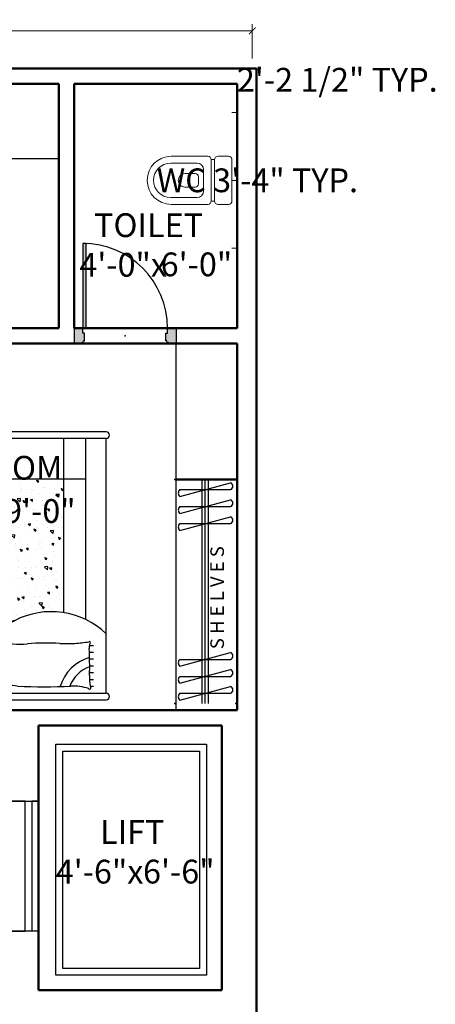
# Model space of a CAD drawing. Units: inches. Extents: x 4508 to 5907, y 877 to 1592.
# Tile 20 of 20: x 5784 to 5907, y 1298 to 1588. Entities that reach past the tile are written whole.
import ezdxf

# ---------------------------------------------------------------- set-up
doc = ezdxf.new("R2010")
doc.units = ezdxf.units.IN
doc.layers.get('DEFPOINTS').update_dxf_attribs({"color": 8})
for name, color, linetype, lineweight in [('A-ANNO-DIMS', 2, 'Continuous', 18), ('A-DOOR', 4, 'Continuous', 25), ('A-EQPM', 6, 'Continuous', 25), ('A-FLOR-CASE', 30, 'Continuous', 25), ('A-FLOR-FIXT', 8, 'Continuous', 18), ('A-FURN', 24, 'Continuous', 18), ('A-WALL', 7, 'Continuous', 50)]:
    doc.layers.add(name, color=color, linetype=linetype, lineweight=lineweight)
doc.layers.add('doors & windows', color=30, linetype='Continuous')
doc.layers.add('furniture', color=24, linetype='Continuous')
doc.styles.get("Standard").update_dxf_attribs({"font": 'arial.ttf'})
doc.dimstyles.new('details', dxfattribs={"dimtxt": 5, "dimasz": 2, "dimexe": 2, "dimexo": 3, "dimgap": 1, "dimtad": 0, "dimdec": 1, "dimzin": 0, "dimdsep": 46, "dimlunit": 4, "dimtxsty": 'Standard', "dimblk": 'ARCHTICK', "dimcen": 3, "dimclrd": 256, "dimclre": 256, "dimclrt": 256, "dimadec": 0, "dimazin": 0, "dimtfac": 0.5, "dimtdec": 1, "dimtofl": 0, "dimtmove": 0, "dimatfit": 3, "dimldrblk": 'CLOSEDBLANK', "dimfxl": 2, "dimtolj": 1, "dimtzin": 0, "dimlwd": -1, "dimlwe": -1, "dimarcsym": 0})
doc.dimstyles.new('text', dxfattribs={"dimtxt": 7, "dimasz": 0, "dimexe": 3, "dimexo": 3, "dimgap": 0, "dimtad": 1, "dimtih": 1, "dimtoh": 1, "dimzin": 3, "dimdsep": 46, "dimlunit": 4, "dimtxsty": 'Standard', "dimblk": 'CLOSEDBLANK', "dimcen": 3, "dimse1": 1, "dimse2": 1, "dimsd1": 1, "dimsd2": 1, "dimclrd": 256, "dimclre": 256, "dimclrt": 256, "dimadec": 0, "dimazin": 0, "dimtfac": 0.5, "dimtofl": 0, "dimtmove": 0, "dimatfit": 3, "dimfxl": 3, "dimtolj": 1, "dimtzin": 0, "dimlwd": -1, "dimlwe": -1, "dimarcsym": 0})

# ---------------------------------------------------------------- blocks, each defined once
blk = doc.blocks.new('*D115')
at = {"layer": 'DEFPOINTS', "color": 0, "transparency": 16777216}
for p in [(5789.99, 1344.38), (5843.99, 1341.42), (5843.99, 1333.76)]:
    blk.add_point(p, dxfattribs=at)
at = {"layer": 'A-ANNO-DIMS', "color": 0, "transparency": 16777216, "insert": (5807.95, 1343.17), "char_height": 7, "attachment_point": 5}
blk.add_mtext('\\A1;         LIFT\\P4\'-6"x', dxfattribs=at)
blk = doc.blocks.new('_ClosedBlank')
at = {"color": 0, "lineweight": -2}
for p, q in [((-1, 0.17), (0, 0)), ((-1, 0.17), (-1, -0.17)), ((0, 0), (-1, -0.17))]:
    blk.add_line(p, q, dxfattribs=at)
blk = doc.blocks.new('*D116')
at = {"layer": 'DEFPOINTS', "color": 0, "transparency": 16777216}
for p in [(5831.31, 1380.42), (5833.5, 1380.42), (5832.34, 1302.42)]:
    blk.add_point(p, dxfattribs=at)
at = {"layer": 'A-ANNO-DIMS', "color": 0, "transparency": 16777216, "insert": (5831.31, 1337.35), "char_height": 7, "attachment_point": 5}
blk.add_mtext('\\A1;6\'-6"', dxfattribs=at)
blk = doc.blocks.new('*D117')
at = {"layer": 'DEFPOINTS', "color": 0, "transparency": 16777216}
for p in [(5791.67, 1535.67), (5698.68, 1533.69), (5791.67, 1523.15)]:
    blk.add_point(p, dxfattribs=at)
at = {"layer": 'A-ANNO-DIMS', "color": 0, "transparency": 16777216, "insert": (5735.91, 1532.61), "char_height": 7, "attachment_point": 5}
blk.add_mtext('\\A1;       KITCHEN\\P7\'-9"x', dxfattribs=at)
blk = doc.blocks.new('commode')
for p, q in [((-7.09, 19.41), (-7.09, 8.61)), ((-5.09, 11.81), (-5.09, 19.57)), ((5.09, 11.81), (5.09, 19.57)), ((7.09, 19.41), (7.09, 8.61)), ((-2, 12.37), (-2, 15.37)), ((2, 12.37), (2, 15.37)), ((-3.15, 9.87), (3.15, 9.87)), ((-1, 11.37), (1, 11.37)), ((-6.09, 7.61), (6.09, 7.61)), ((-6.09, 6.61), (-6.09, 7.61)), ((-6.09, 6.61), (6.09, 6.61)), ((6.09, 7.61), (6.09, 6.61)), ((-7.09, 2.5), (-7.09, 5.61)), ((7.09, 2.5), (7.09, 5.61)), ((-20, 1.5), (-20, 0)), ((-6.09, 1.5), (6.09, 1.5)), ((0, 1.5), (0, 0)), ((20, 1.5), (20, 0))]:
    blk.add_line(p, q)
for centre, radius, start, end in [((0, 19.41), 7.09, 0, 180), ((0, 19.57), 5.09, 0, 180), ((0, 15.37), 2, 0, 180), ((-3.15, 11.81), 1.94, 180, 270), ((-1, 12.37), 1, 180, 270), ((1, 12.37), 1, 270, 0), ((3.15, 11.81), 1.94, 270, 0), ((-6.09, 8.61), 1, 180, 270), ((-6.09, 5.61), 1, 90, 180), ((6.09, 8.61), 1, 270, 0), ((6.09, 5.61), 1, 0, 90), ((-6.09, 2.5), 1, 180, 270), ((6.09, 2.5), 1, 270, 0)]:
    blk.add_arc(centre, radius, start, end)
blk = doc.blocks.new('*D119')
at = {"layer": 'DEFPOINTS', "color": 0, "transparency": 16777216}
for p in [(5800.49, 1515.06), (5848.49, 1515.63), (5848.49, 1512.47)]:
    blk.add_point(p, dxfattribs=at)
at = {"layer": 'A-ANNO-DIMS', "color": 0, "transparency": 16777216, "insert": (5814.91, 1521.94), "char_height": 7, "attachment_point": 5}
blk.add_mtext('\\A1;       TOILET\\P4\'-0"x', dxfattribs=at)
blk = doc.blocks.new('*D120')
at = {"layer": 'DEFPOINTS', "color": 0, "transparency": 16777216}
for p in [(5827.85, 1569.42), (5836.51, 1569.42), (5824.86, 1497.42)]:
    blk.add_point(p, dxfattribs=at)
at = {"layer": 'A-ANNO-DIMS', "color": 0, "transparency": 16777216, "insert": (5836.51, 1516.23), "char_height": 7, "attachment_point": 5}
blk.add_mtext('\\A1;6\'-0"', dxfattribs=at)
blk = doc.blocks.new('_ArchTick')
at = {"color": 0, "linetype": 'ByBlock', "const_width": 0.15}
blk.add_lwpolyline([(-0.5, -0.5), (0.5, 0.5)], dxfattribs=at)
blk = doc.blocks.new('*D121')
at = {"layer": 'A-ANNO-DIMS', "color": 0, "transparency": 16777216}
for p, q in [((5573.99, 1576.92), (5573.99, 1587.03)), ((5852.99, 1576.92), (5852.99, 1587.03)), ((5573.99, 1585.03), (5703.86, 1585.03)), ((5852.99, 1585.03), (5723.12, 1585.03))]:
    blk.add_line(p, q, dxfattribs=at)
at = {"layer": 'DEFPOINTS', "color": 0, "transparency": 16777216}
for p in [(5852.99, 1585.03), (5573.99, 1573.92), (5852.99, 1573.92)]:
    blk.add_point(p, dxfattribs=at)
at = {"layer": 'A-ANNO-DIMS', "color": 0, "transparency": 16777216, "xscale": 2, "yscale": 2, "zscale": 2, "rotation": 180}
blk.add_blockref('_ArchTick', (5573.99, 1585.03), dxfattribs=at)
at = {"layer": 'A-ANNO-DIMS', "color": 0, "transparency": 16777216, "xscale": 2, "yscale": 2, "zscale": 2}
blk.add_blockref('_ArchTick', (5852.99, 1585.03), dxfattribs=at)
at = {"layer": 'A-ANNO-DIMS', "color": 0, "transparency": 16777216, "insert": (5713.49, 1585.03), "char_height": 5, "attachment_point": 5}
blk.add_mtext('\\A1;23\'-3"', dxfattribs=at)
blk = doc.blocks.new('*D123')
at = {"layer": 'DEFPOINTS', "color": 0, "transparency": 16777216}
for p in [(5792.26, 1492.92), (5759.25, 1384.92), (5790.34, 1384.92)]:
    blk.add_point(p, dxfattribs=at)
at = {"layer": 'A-ANNO-DIMS', "color": 0, "transparency": 16777216, "insert": (5790.34, 1443.57), "char_height": 7, "attachment_point": 5}
blk.add_mtext('\\A1;9\'-0"', dxfattribs=at)
blk = doc.blocks.new('*D124')
at = {"layer": 'DEFPOINTS', "color": 0, "transparency": 16777216}
for p in [(5715.67, 1442.67), (5861.17, 1442.67), (5861.17, 1439.77)]:
    blk.add_point(p, dxfattribs=at)
at = {"layer": 'A-ANNO-DIMS', "color": 0, "transparency": 16777216, "insert": (5764.12, 1449.77), "char_height": 7, "attachment_point": 5}
blk.add_mtext('\\A1;        BED ROOM\\P12\'-1{\\H0.5x;\\S1/2;}"x', dxfattribs=at)
blk = doc.blocks.new('bed')
at = {"layer": 'furniture'}
h = blk.add_hatch(dxfattribs=at)
h.set_pattern_fill('AR-CONC', color=256, angle=-90, style=0)
h.set_pattern_definition([(320, (0, 2.38), (-0.6275, -7.1726), [0.75, -8.25]), (265, (0, 2.38), (7.5219, 1.3875), [0.6, -6.6]), (10.451, (-0.052, 1.782), (6.8944, -5.7851), [0.6374, -7.0114]), (316.184, (2, 2.38), (-1.6552, -10.6724), [1.125, -12.375]), (6.636, (1.862, 1.491), (9.7412, -9.3466), [0.9561, -10.5171]), (261.184, (2, 2.38), (9.7412, -9.3466), [0.9, -9.9]), (291, (1.5, 1.38), (-4.0262, -5.96907), [0.75, -8.25]), (236, (1.5, 1.38), (7.2515, -2.43315), [0.6, -6.6]), (341.451, (1.1645, 0.8826), (3.2253, -8.4022), [0.6374, -7.0114]), (307.5, (0, 2.38), (3.32894, -0.1216), [0, -6.52, 0, -6.7, 0, -6.625]), (277.5, (0, 2.38), (3.94412, -2.6307), [0, -3.82, 0, -6.37, 0, -2.525]), (237.5, (0, 4.61), (-0.22555, -5.33822), [0, -2.5, 0, -7.8, 0, -10.35]), (227.5, (0, 5.61), (1.00105, -5.83186), [0, -3.25, 0, -5.18, 0, -7.35])])
h.paths.add_polyline_path([(30.01, -68), (30.01, -26.5, 0.263043), (23.9, -35.15, 0.293424), (-9.18, -26.47, -0.156683), (-23.39, -28.72), (-23.39, -68)])
for p, q in [((0, -3), (0, 0)), ((36.01, -3), (-36.01, -3)), ((-36.01, -5), (-36.01, -80)), ((36.01, -5), (-36.01, -5)), ((0, -8), (0, -5)), ((36.01, -80), (36.01, -5)), ((-31.24, -7.07), (-32.24, -7.07)), ((-3.81, -7.07), (-2.81, -7.07)), ((3.89, -7.07), (2.89, -7.07)), ((31.63, -7.07), (32.63, -7.07)), ((-31.24, -9.07), (-32.24, -9.07)), ((-31.24, -11.07), (-32.24, -11.07)), ((-3.81, -9.07), (-2.81, -9.07)), ((-3.81, -11.07), (-2.81, -11.07)), ((3.89, -9.07), (2.89, -9.07)), ((3.89, -11.07), (2.89, -11.07)), ((31.63, -9.07), (32.63, -9.07)), ((31.63, -11.07), (32.63, -11.07)), ((-31.24, -13.07), (-32.24, -13.07)), ((-3.81, -13.07), (-2.81, -13.07)), ((3.89, -13.07), (2.89, -13.07)), ((31.63, -13.07), (32.63, -13.07)), ((-31.24, -15.07), (-32.24, -15.07)), ((-31.24, -17.07), (-32.24, -17.07)), ((-3.81, -15.07), (-2.81, -15.07)), ((-3.81, -17.07), (-2.81, -17.07)), ((3.89, -15.07), (2.89, -15.07)), ((3.89, -17.07), (2.89, -17.07)), ((31.63, -15.07), (32.63, -15.07)), ((31.63, -17.07), (32.63, -17.07)), ((-31.24, -19.07), (-32.24, -19.07)), ((-3.81, -19.07), (-2.81, -19.07)), ((3.89, -19.07), (2.89, -19.07)), ((31.63, -19.07), (32.63, -19.07)), ((-36.01, -80), (36.01, -80)), ((-36.01, -82), (36.01, -82))]:
    blk.add_line(p, q, dxfattribs=at)
at = {"layer": 'furniture', "ltscale": 5}
blk.add_line((-30.01, -26.66), (-30.01, -80), dxfattribs=at)
at = {"layer": 'furniture', "ltscale": 0.3}
for p, q in [((-23.39, -80), (-23.39, -28.72)), ((-30.01, -68), (30.01, -68))]:
    blk.add_line(p, q, dxfattribs=at)
at = {"layer": 'furniture', "ltscale": 7}
blk.add_line((30.01, -80), (30.01, -26.5), dxfattribs=at)
at = {"layer": 'furniture'}
for centre, radius, start, end in [((-35.95, -4), 1, 93.3831, 266.6169), ((35.95, -4), 1, 273.3831, 86.6169), ((-31.1, -6.57), 0.382, 35.8976, 208.6272), ((-44.44, -13.85), 14.82, 27.1629, 28.6272), ((-46.76, -9.65), 15.72, 357.4804, 9.3956), ((-34.45, -3.51), 9.85, 289.8695, 338.9843), ((-34.45, -3.51), 12.47, 286.0319, 344.1205), ((-26.35, 6.68), 13.76, 251.1782, 273.3982), ((-18.02, -163.6), 156.72, 87.0032, 92.7497), ((-8.03, 2.03), 9.29, 258.896, 294.7184), ((0.25, -8.8), 4.49, 159.0146, 186.273), ((-4.03, -6.67), 0.282, 335.7259, 114.303), ((3.22, -9.94), 7.68, 155.7259, 159.0146), ((4.11, -6.67), 0.282, 65.697, 204.2741), ((-3.14, -9.94), 7.68, 20.9854, 24.2741), ((-0.17, -8.8), 4.49, 353.727, 20.9854), ((8.12, 2.03), 9.29, 245.2816, 281.104), ((18.1, -163.6), 156.72, 87.2503, 92.9968), ((34.54, -3.51), 12.47, 195.8795, 253.9681), ((34.54, -3.51), 9.85, 201.0157, 250.1305), ((26.43, 6.68), 13.76, 266.6018, 288.8218), ((31.18, -6.57), 0.382, 331.3728, 144.1024), ((46.84, -9.65), 15.72, 170.6044, 182.5196), ((44.53, -13.85), 14.82, 151.3728, 152.8371), ((-28.62, 31.03), 42.31, 266.4836, 266.6487), ((54.88, -13.16), 85.99, 178.1209, 183.3613), ((-32.82, -12.44), 28.78, 354.3784, 6.273), ((32.9, -12.44), 28.78, 173.727, 185.6216), ((-54.8, -13.16), 85.99, 356.6387, 1.8791), ((28.7, 31.03), 42.31, 273.3513, 273.5164), ((12.28, -16.11), 16.48, 177.0317, 192.8678), ((-12.19, -16.11), 16.48, 347.1322, 2.9683), ((-31.05, -19.91), 0.291, 147.6219, 311.9343), ((-33.2, -18.55), 2.25, 327.6219, 339.2246), ((-34.13, -18.41), 3.18, 342.7809, 3.755), ((-24.4, -58.01), 38.42, 93.5164, 99.6766), ((-24.52, -56.06), 36.48, 86.4836, 93.5164), ((-18.49, 70.49), 90.23, 267.5921, 273.6329), ((-10.31, -44.95), 25.52, 75.952, 95.5452), ((-3.95, -19.99), 0.265, 231.9005, 52.8902), ((4.03, -19.99), 0.265, 127.1098, 308.0995), ((7.57, -34.68), 14.87, 87.3976, 103.1191), ((11.44, -34.81), 15.32, 84.694, 102.0355), ((18.57, 70.49), 90.23, 266.3671, 272.4079), ((24.6, -56.06), 36.48, 86.4836, 93.5164), ((24.48, -58.01), 38.42, 80.3234, 86.4836), ((31.13, -19.91), 0.291, 228.0657, 32.3781), ((34.21, -18.41), 3.18, 176.245, 197.2191), ((33.28, -18.55), 2.25, 200.7754, 212.3781), ((-19.79, -5.47), 23.53, 226.4061, 297.4441), ((12.51, -69.71), 48.38, 60.9345, 116.3227), ((0.6, -56.57), 31.65, 42.5874, 108.5034), ((34.61, -36.23), 10.76, 101.1719, 174.259), ((-35.95, -81), 1, 93.3831, 266.6169), ((35.95, -81), 1, 273.3831, 86.6169)]:
    blk.add_arc(centre, radius, start, end, dxfattribs=at)
blk = doc.blocks.new('hangers')
at = {"layer": 'furniture'}
for p, q in [((1, 7.5), (5, -7.5)), ((3, 7.5), (3, -7.5)), ((6, 7.5), (10, -7.5)), ((8, 7.5), (8, -7.5)), ((11, 7.5), (15, -7.5)), ((13, 7.5), (13, -7.5)), ((51, 7.5), (55, -7.5)), ((53, 7.5), (53, -7.5)), ((56, 7.5), (60, -7.5)), ((58, 7.5), (58, -7.5)), ((61, 7.5), (65, -7.5)), ((63, 7.5), (63, -7.5)), ((66, 1), (0, 1)), ((0, 0), (66, 0)), ((0, -1), (66, -1))]:
    blk.add_line(p, q, dxfattribs=at)
for centre, radius, start, end in [((2, 6.62), 1.33, 41.2884, 138.7116), ((7, 6.62), 1.33, 41.2884, 138.7116), ((12, 6.62), 1.33, 41.2884, 138.7116), ((52, 6.62), 1.33, 41.2884, 138.7116), ((57, 6.62), 1.33, 41.2884, 138.7116), ((62, 6.62), 1.33, 41.2884, 138.7116), ((4, -7.08), 1.08, 202.5549, 337.4451), ((9, -7.08), 1.08, 202.5549, 337.4451), ((14, -7.08), 1.08, 202.5549, 337.4451), ((54, -7.08), 1.08, 202.5549, 337.4451), ((59, -7.08), 1.08, 202.5549, 337.4451), ((64, -7.08), 1.08, 202.5549, 337.4451)]:
    blk.add_arc(centre, radius, start, end, dxfattribs=at)
for p in [(0, 9), (66, 9), (0, -9), (66, -9)]:
    blk.add_point(p, dxfattribs=at)
blk.add_text('S H E L V E S', height=4, dxfattribs=at).set_placement((16, -5.52))
blk = doc.blocks.new('D2')
at = {"layer": 'doors & windows'}
h = blk.add_hatch(dxfattribs=at)
h.set_pattern_fill('DOTS', color=256, scale=2, angle=180, style=0)
h.set_pattern_definition([(180, (0, -4), (-0.0625, -0.125), [0, -0.125])])
h.paths.add_polyline_path([(2.5, 0), (3.5, 0), (3.5, 24.98, 0.010003), (2.5, 25)])
h = blk.add_hatch(dxfattribs=at)
h.set_pattern_fill('DOTS', color=256, scale=2, angle=180, style=0)
h.set_pattern_definition([(180, (0, 0), (-0.0625, -0.125), [0, -0.125])])
edge = h.paths.add_edge_path()
edge.add_line((27.5, 0), (27.5, -1.5))
edge.add_line((27.5, -1.5), (27, -1.5))
edge.add_line((27, -1.5), (27, -3.75))
edge.add_line((27, -3.75), (27.25, -3.75))
edge.add_arc((27.76, -3.74), 0.509, 181.0059, 268.9941)
edge.add_line((27.75, -4.25), (27.75, -4.5))
edge.add_line((27.75, -4.5), (30, -4.5))
edge.add_line((30, -4.5), (30, 0))
edge.add_line((30, 0), (27.5, 0))
edge = h.paths.add_edge_path()
edge.add_line((2.5, -1.5), (2.5, 0))
edge.add_line((2.5, 0), (0, 0))
edge.add_line((0, 0), (0, -4.5))
edge.add_line((0, -4.5), (2.25, -4.5))
edge.add_line((2.25, -4.5), (2.25, -4.25))
edge.add_arc((2.24, -3.74), 0.509, 271.0059, 358.9941)
edge.add_line((2.75, -3.75), (3, -3.75))
edge.add_line((3, -3.75), (3, -1.5))
edge.add_line((3, -1.5), (2.5, -1.5))
for p, q in [((0, 0), (0, -4.5)), ((30, 0), (30, -4.5))]:
    blk.add_line(p, q)
blk.add_lwpolyline([(3.5, 0), (3.5, 25), (2.5, 25), (2.5, 0)], close=True, dxfattribs=at)
for points in [[(3, -3.75), (3, -1.5), (2.5, -1.5), (2.5, 0), (0, 0)], [(27, -3.75), (27, -1.5), (27.5, -1.5), (27.5, 0), (30, 0)], [(0, -4.5), (2.25, -4.5)], [(30, -4.5), (27.75, -4.5)]]:
    blk.add_lwpolyline(points, dxfattribs=at)
for points in [[(2.25, -4.5), (2.25, -4.25, 0.403966), (2.75, -3.75), (3, -3.75)], [(27.75, -4.5), (27.75, -4.25, -0.403966), (27.25, -3.75), (27, -3.75)]]:
    blk.add_lwpolyline(points, format="xyb", dxfattribs=at)
at = {"layer": 'doors & windows', "ltscale": 6}
blk.add_arc((2.5, 0), 25, 0, 90, dxfattribs=at)
at = {"layer": 'doors & windows'}
blk.add_point((15, -2.25), dxfattribs=at)
blk = doc.blocks.new('*D154')
at = {"layer": 'DEFPOINTS', "color": 0, "transparency": 16777216}
for p in [(5848.49, 1560.99), (5854.49, 1560.99), (5848.49, 1520.99)]:
    blk.add_point(p, dxfattribs=at)
at = {"layer": 'A-ANNO-DIMS', "transparency": 16777216, "insert": (5854.49, 1540.99), "char_height": 7, "attachment_point": 5}
blk.add_mtext('\\A1;WC 3\'-4" TYP.', dxfattribs=at)
blk = doc.blocks.new('*D155')
at = {"layer": 'DEFPOINTS', "color": 0, "transparency": 16777216}
for p in [(5821.99, 1566.99), (5821.99, 1560.99), (5848.49, 1560.99)]:
    blk.add_point(p, dxfattribs=at)
at = {"layer": 'A-ANNO-DIMS', "transparency": 16777216, "insert": (5878.04, 1570.61), "char_height": 7, "attachment_point": 5}
blk.add_mtext('\\A1;2\'-2 1/2" TYP.', dxfattribs=at)
blk = doc.blocks.new('*D194')
at = {"layer": 'DEFPOINTS', "color": 0, "transparency": 16777216}
for p in [(5854.266243, 1573.916611), (5890.541519, 1573.916611), (5855.991519, 925.916611)]:
    blk.add_point(p, dxfattribs=at)
at = {"layer": 'A-ANNO-DIMS', "transparency": 16777216, "insert": (5890.541519, 1249.916611), "char_height": 7, "attachment_point": 5}
blk.add_mtext('\\A1;54\'-0"', dxfattribs=at)

msp = doc.modelspace()

# ---------------------------------------------------------------- linework, layer by layer
at = {"layer": 'A-EQPM'}
for points in [[(5795.092, 1374.867), (5839.445, 1374.867), (5839.445, 1306.802), (5795.092, 1306.802)], [(5797.092, 1372.867), (5837.445, 1372.867), (5837.445, 1308.802), (5797.092, 1308.802)]]:
    msp.add_lwpolyline(points, close=True, dxfattribs=at)
msp.add_lwpolyline([(5789.989, 1319.79), (5780.989, 1319.79), (5785.989, 1319.79), (5785.989, 1358.075), (5780.989, 1358.075), (5789.989, 1358.075), (5787.989, 1358.075), (5787.989, 1319.79)], dxfattribs=at)
at = {"layer": 'A-FLOR-CASE'}
for p, q in [((5698.511, 1547.417), (5795.989, 1547.417)), ((5830.489, 1384.917), (5830.489, 1492.917))]:
    msp.add_line(p, q, dxfattribs=at)
at = {"layer": 'A-WALL'}
for p, q in [((5573.989, 1573.917), (5854.266, 1573.917)), ((5854.266, 1573.917), (5854.266, 1298.576)), ((5698.511, 1569.417), (5795.989, 1569.417)), ((5795.989, 1569.417), (5795.989, 1497.417)), ((5800.489, 1569.417), (5848.489, 1569.417)), ((5800.489, 1569.417), (5800.489, 1497.417)), ((5848.489, 1569.417), (5848.489, 1497.417)), ((5694.344, 1497.417), (5795.989, 1497.417)), ((5800.489, 1497.417), (5848.489, 1497.417)), ((5698.865, 1492.917), (5848.489, 1492.917)), ((5848.489, 1492.917), (5848.489, 1384.917)), ((5830.489, 1452.867), (5848.489, 1452.867)), ((5699.365, 1384.917), (5848.489, 1384.917)), ((5789.989, 1380.417), (5789.989, 1302.417)), ((5789.989, 1380.417), (5843.989, 1380.417)), ((5843.989, 1380.417), (5843.989, 1302.417)), ((5789.989, 1302.417), (5843.989, 1302.417)), ((5855.992, 925.917), (5854.266, 1298.576))]:
    msp.add_line(p, q, dxfattribs=at)

# ---------------------------------------------------------------- block references
at = {"layer": 'A-DOOR'}
msp.add_blockref('D2', (5800.489, 1497.417), dxfattribs=at)
at = {"layer": 'A-FLOR-FIXT', "rotation": 90}
msp.add_blockref('commode', (5848.489, 1540.987), dxfattribs=at)
at = {"layer": 'A-FURN'}
for name, p, rotation in [('bed', (5773.927, 1384.917), 180), ('hangers', (5839.101, 1386.867), 90)]:
    msp.add_blockref(name, p, dxfattribs=dict(at, rotation=rotation))

# ---------------------------------------------------------------- dimensions: what is measured, and where the dimension line sits
at = {"layer": 'A-ANNO-DIMS'}
dim = msp.add_linear_dim(base=(5852.989, 1585.029), p1=(5573.989, 1573.917), p2=(5852.989, 1573.917), dimstyle='details', override={"dimclrd": 0, "dimclre": 0, "dimclrt": 0}, dxfattribs=at)
dim.commit()
dim.dimension.update_dxf_attribs({"geometry": '*D121', "text_midpoint": (5713.489, 1585.029)})
for base, p1, p2, angle, text, picture, middle in [((5821.989, 1566.987), (5848.489, 1560.987), (5821.989, 1560.987), 180, '<> TYP.', '*D155', (5878.038, 1570.607)), ((5854.489, 1560.987), (5848.489, 1520.987), (5848.489, 1560.987), 90, 'WC <> TYP.', '*D154', (5854.489, 1540.987))]:
    dim = msp.add_linear_dim(base=base, p1=p1, p2=p2, angle=angle, text=text, dimstyle='text', override={"dimdec": 1, "dimrnd": 0, "dimzin": 1, "dimlunit": 4, "dimfrac": 2}, dxfattribs=at)
    dim.commit()
    dim.dimension.update_dxf_attribs({"geometry": picture, "text_midpoint": middle})
dim = msp.add_linear_dim(base=(5890.542, 1573.917), p1=(5855.992, 925.917), p2=(5854.266, 1573.917), angle=90, dimstyle='text', override={"dimdec": 1, "dimlfac": 1, "dimrnd": 0, "dimzin": 1, "dimdsep": 46, "dimlunit": 4, "dimfrac": 2}, dxfattribs=at)
dim.commit()
dim.dimension.update_dxf_attribs({"geometry": '*D194', "text_midpoint": (5890.542, 1249.917)})
for base, p1, p2, angle, picture, middle in [((5836.513, 1569.417), (5824.861, 1497.417), (5827.851, 1569.417), 90, '*D120', (5836.513, 1516.229)), ((5790.337, 1384.917), (5792.265, 1492.917), (5759.245, 1384.917), 90, '*D123', (5790.337, 1443.573)), ((5831.313, 1380.417), (5832.342, 1302.417), (5833.497, 1380.417), 270, '*D116', (5831.313, 1337.346))]:
    dim = msp.add_linear_dim(base=base, p1=p1, p2=p2, angle=angle, dimstyle='text', override={"dimclrd": 0, "dimclre": 0, "dimclrt": 0}, dxfattribs=at)
    dim.commit()
    dim.dimension.update_dxf_attribs({"geometry": picture, "text_midpoint": middle, "dimtype": 160})
for base, p1, p2, text, picture, middle in [((5791.668, 1523.146), (5698.676, 1533.691), (5791.668, 1535.667), '       KITCHEN\\P<>x', '*D117', (5735.911, 1523.146)), ((5848.489, 1512.472), (5800.489, 1515.065), (5848.489, 1515.633), '       TOILET\\P<>x', '*D119', (5814.914, 1512.472)), ((5861.167, 1439.773), (5715.667, 1442.667), (5861.167, 1442.667), '        BED ROOM\\P<>x', '*D124', (5764.115, 1439.773)), ((5843.989, 1333.764), (5789.989, 1344.375), (5843.989, 1341.417), '         LIFT\\P<>x', '*D115', (5807.947, 1333.764))]:
    dim = msp.add_linear_dim(base=base, p1=p1, p2=p2, text=text, dimstyle='text', override={"dimclrd": 0, "dimclre": 0, "dimclrt": 0}, dxfattribs=at)
    dim.commit()
    dim.dimension.update_dxf_attribs({"geometry": picture, "text_midpoint": middle, "dimtype": 160})

doc.saveas('drawing.dxf')
